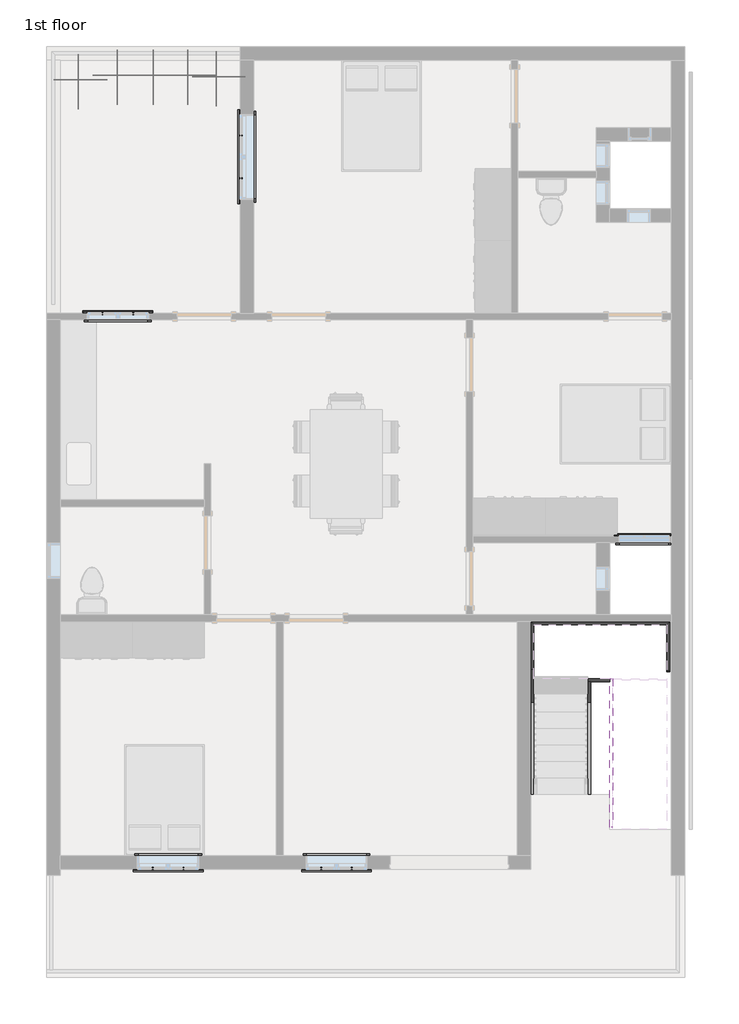
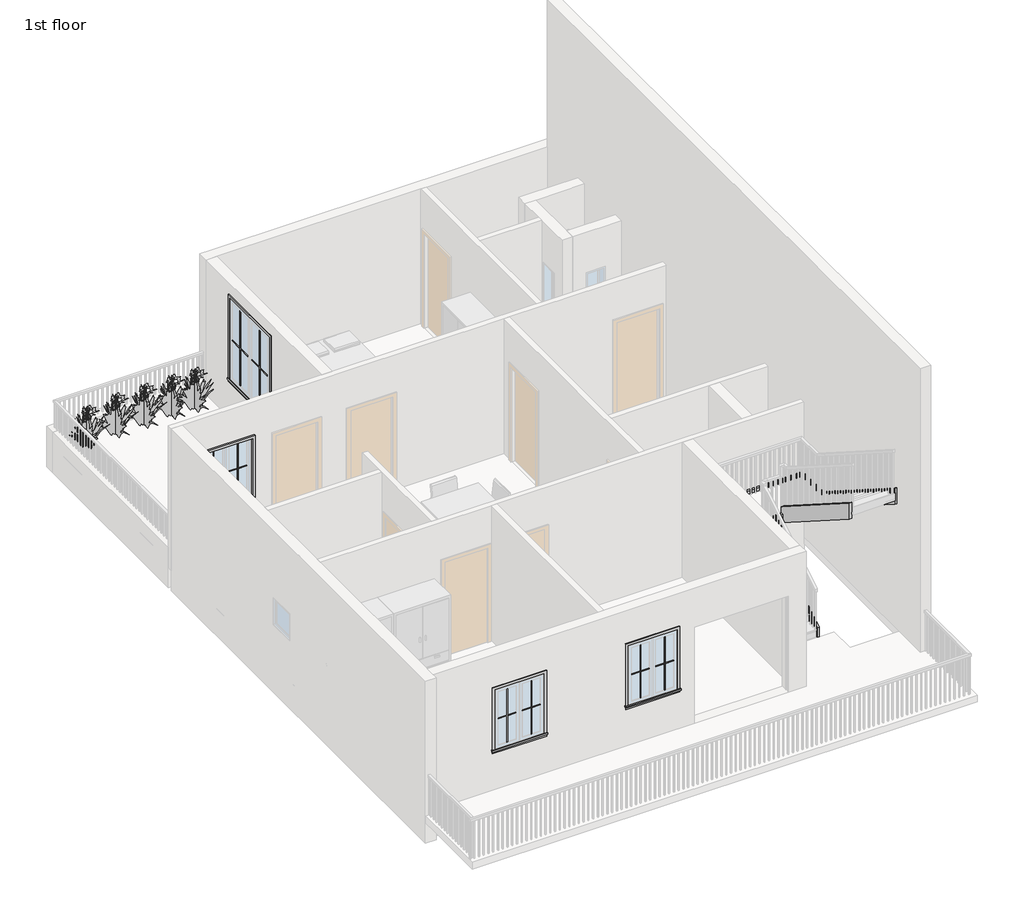
# One storey, part 5 of 5: 20 proxies, 8 members, 5 geographic elements.
"""IFC4 building model written with IfcOpenShell, lengths in millimetres."""

from ifc_helpers import new_model, si_unit, frame, origin, place, context, project, spatial, polyline, outline, extrude, faceted_brep, transform, mapped, element, save
from components import muntin_pattern_2x2_muntin_pattern_2x2_bff912c5, muntin_pattern_2x2_muntin_pattern_2x2_c2194282, muntin_pattern_2x2_muntin_pattern_2x2_88bf7f41, muntin_pattern_2x2_muntin_pattern_2x2_3dfd0a47, muntin_pattern_2x2_muntin_pattern_2x2_b3fe6957, muntin_pattern_2x2_muntin_pattern_2x2_3e0ecaf2, trim_window_exterior_flat_with_sill_e04b3088, trim_window_exterior_flat_with_sill_4930676f, trim_window_exterior_flat_with_sill_41619996, trim_window_interior_flat_picture_frame_2a7685fe, trim_window_interior_flat_picture_frame_dd064338, trim_window_interior_flat_picture_frame_51c85655, rpc_plant_tropical_55f6ff97

model = new_model("IFC4")

# Units and contexts
model_context = context("Model", 3, world=origin())
ifc_project = project(units=[si_unit("LENGTHUNIT", "METRE", prefix="MILLI")], contexts=[model_context])

# Site, building, storey
site = spatial("IfcSite", under=ifc_project)
building = spatial("IfcBuilding", under=site)
storey = spatial("IfcBuildingStorey", under=building, Name="1st floor", Elevation=3810.0)

# Proxies
placement = place(None, origin())
muntin_pattern_2x2_muntin_pattern_2x2_shape = muntin_pattern_2x2_muntin_pattern_2x2_bff912c5(model_context)
element("IfcBuildingElementProxy", 1, Name="Muntin Pattern_2x2 : Muntin Pattern_2x2", ObjectType="Muntin Pattern_2x2 : Muntin Pattern_2x2", at=placement, inside=storey, context=model_context, shape_type="MappedRepresentation", body=[
    mapped(muntin_pattern_2x2_muntin_pattern_2x2_shape, transform((-4824.2248597, 10579.5632925, 4794.25), x_axis=(0.0, 1.0, 0.0), y_axis=(-1.0, 0.0, 0.0), z_axis=(0.0, 0.0, 1.0))),
])
muntin_pattern_2x2_muntin_pattern_2x2_2_shape = muntin_pattern_2x2_muntin_pattern_2x2_c2194282(model_context)
element("IfcBuildingElementProxy", 2, Name="Muntin Pattern_2x2 : Muntin Pattern_2x2", ObjectType="Muntin Pattern_2x2 : Muntin Pattern_2x2", at=placement, inside=storey, context=model_context, shape_type="MappedRepresentation", body=[
    mapped(muntin_pattern_2x2_muntin_pattern_2x2_2_shape, transform((-4824.2248597, 11300.2882925, 4794.25), x_axis=(0.0, -1.0, 0.0), y_axis=(1.0, 0.0, 0.0), z_axis=(0.0, 0.0, 1.0))),
])
muntin_pattern_2x2_muntin_pattern_2x2_3_shape = muntin_pattern_2x2_muntin_pattern_2x2_88bf7f41(model_context)
element("IfcBuildingElementProxy", 3, Name="Muntin Pattern_2x2 : Muntin Pattern_2x2", ObjectType="Muntin Pattern_2x2 : Muntin Pattern_2x2", at=placement, inside=storey, context=model_context, shape_type="MappedRepresentation", body=[
    mapped(muntin_pattern_2x2_muntin_pattern_2x2_3_shape, transform((-7162.6123597, 8288.8007925, 4794.25), x_axis=(1.0, 0.0, 0.0), y_axis=(0.0, 1.0, 0.0), z_axis=(0.0, 0.0, 1.0))),
])
element("IfcBuildingElementProxy", 4, Name="Muntin Pattern_2x2 : Muntin Pattern_2x2", ObjectType="Muntin Pattern_2x2 : Muntin Pattern_2x2", at=placement, inside=storey, context=model_context, shape_type="MappedRepresentation", body=[
    mapped(muntin_pattern_2x2_muntin_pattern_2x2_3_shape, transform((-5794.1873597, -1102.8492075, 4794.25), x_axis=(-1.0, 0.0, 0.0), y_axis=(0.0, -1.0, 0.0), z_axis=(0.0, 0.0, 1.0))),
])
element("IfcBuildingElementProxy", 5, Name="Muntin Pattern_2x2 : Muntin Pattern_2x2", ObjectType="Muntin Pattern_2x2 : Muntin Pattern_2x2", at=placement, inside=storey, context=model_context, shape_type="MappedRepresentation", body=[
    mapped(muntin_pattern_2x2_muntin_pattern_2x2_3_shape, transform((-2946.0873597, -1102.8492075, 4794.25), x_axis=(-1.0, 0.0, 0.0), y_axis=(0.0, -1.0, 0.0), z_axis=(0.0, 0.0, 1.0))),
])
muntin_pattern_2x2_muntin_pattern_2x2_4_shape = muntin_pattern_2x2_muntin_pattern_2x2_3dfd0a47(model_context)
element("IfcBuildingElementProxy", 6, Name="Muntin Pattern_2x2 : Muntin Pattern_2x2", ObjectType="Muntin Pattern_2x2 : Muntin Pattern_2x2", at=placement, inside=storey, context=model_context, shape_type="MappedRepresentation", body=[
    mapped(muntin_pattern_2x2_muntin_pattern_2x2_4_shape, transform((-6645.0873597, 8288.8007925, 4794.25), x_axis=(-1.0, 0.0, 0.0), y_axis=(0.0, -1.0, 0.0), z_axis=(0.0, 0.0, 1.0))),
])
element("IfcBuildingElementProxy", 7, Name="Muntin Pattern_2x2 : Muntin Pattern_2x2", ObjectType="Muntin Pattern_2x2 : Muntin Pattern_2x2", at=placement, inside=storey, context=model_context, shape_type="MappedRepresentation", body=[
    mapped(muntin_pattern_2x2_muntin_pattern_2x2_4_shape, transform((-6311.7123597, -1102.8492075, 4794.25), x_axis=(1.0, 0.0, 0.0), y_axis=(0.0, 1.0, 0.0), z_axis=(0.0, 0.0, 1.0))),
])
element("IfcBuildingElementProxy", 8, Name="Muntin Pattern_2x2 : Muntin Pattern_2x2", ObjectType="Muntin Pattern_2x2 : Muntin Pattern_2x2", at=placement, inside=storey, context=model_context, shape_type="MappedRepresentation", body=[
    mapped(muntin_pattern_2x2_muntin_pattern_2x2_4_shape, transform((-3463.6123597, -1102.8492075, 4794.25), x_axis=(1.0, 0.0, 0.0), y_axis=(0.0, 1.0, 0.0), z_axis=(0.0, 0.0, 1.0))),
])
muntin_pattern_2x2_muntin_pattern_2x2_5_shape = muntin_pattern_2x2_muntin_pattern_2x2_b3fe6957(model_context)
element("IfcBuildingElementProxy", 9, Name="Muntin Pattern_2x2 : Muntin Pattern_2x2", ObjectType="Muntin Pattern_2x2 : Muntin Pattern_2x2", at=placement, inside=storey, context=model_context, shape_type="MappedRepresentation", body=[
    mapped(muntin_pattern_2x2_muntin_pattern_2x2_5_shape, transform((1784.5376403, 4516.9007925, 4184.65), x_axis=(1.0, 0.0, 0.0), y_axis=(0.0, 1.0, 0.0), z_axis=(0.0, 0.0, 1.0))),
])
muntin_pattern_2x2_muntin_pattern_2x2_6_shape = muntin_pattern_2x2_muntin_pattern_2x2_3e0ecaf2(model_context)
element("IfcBuildingElementProxy", 10, Name="Muntin Pattern_2x2 : Muntin Pattern_2x2", ObjectType="Muntin Pattern_2x2 : Muntin Pattern_2x2", at=placement, inside=storey, context=model_context, shape_type="MappedRepresentation", body=[
    mapped(muntin_pattern_2x2_muntin_pattern_2x2_6_shape, transform((2213.1626403, 4516.9007925, 4184.65), x_axis=(-1.0, 0.0, 0.0), y_axis=(0.0, -1.0, 0.0), z_axis=(0.0, 0.0, 1.0))),
])
trim_window_exterior_flat_with_sill_shape = trim_window_exterior_flat_with_sill_e04b3088(model_context)
element("IfcBuildingElementProxy", 11, Name="Trim-Window-Exterior-Flat : with Sill", ObjectType="Trim-Window-Exterior-Flat : with Sill", at=placement, inside=storey, context=model_context, shape_type="MappedRepresentation", body=[
    mapped(trim_window_exterior_flat_with_sill_shape, transform((-4833.7498597, 10939.9257925, 6553.2), x_axis=(0.0, -1.0, 0.0), y_axis=(0.0, 0.0, 1.0), z_axis=(-1.0, 0.0, 0.0))),
])
trim_window_exterior_flat_with_sill_2_shape = trim_window_exterior_flat_with_sill_4930676f(model_context)
element("IfcBuildingElementProxy", 12, Name="Trim-Window-Exterior-Flat : with Sill", ObjectType="Trim-Window-Exterior-Flat : with Sill", at=placement, inside=storey, context=model_context, shape_type="MappedRepresentation", body=[
    mapped(trim_window_exterior_flat_with_sill_2_shape, transform((-6903.8498597, 8298.3257925, 6070.6), x_axis=(-1.0, 0.0, 0.0), y_axis=(0.0, 0.0, 1.0), z_axis=(0.0, 1.0, 0.0))),
])
element("IfcBuildingElementProxy", 13, Name="Trim-Window-Exterior-Flat : with Sill", ObjectType="Trim-Window-Exterior-Flat : with Sill", at=placement, inside=storey, context=model_context, shape_type="MappedRepresentation", body=[
    mapped(trim_window_exterior_flat_with_sill_2_shape, transform((-6052.9498597, -1112.3742075, 6070.6), x_axis=(1.0, 0.0, 0.0), y_axis=(0.0, 0.0, 1.0), z_axis=(0.0, -1.0, 0.0))),
])
element("IfcBuildingElementProxy", 14, Name="Trim-Window-Exterior-Flat : with Sill", ObjectType="Trim-Window-Exterior-Flat : with Sill", at=placement, inside=storey, context=model_context, shape_type="MappedRepresentation", body=[
    mapped(trim_window_exterior_flat_with_sill_2_shape, transform((-3204.8498597, -1112.3742075, 6070.6), x_axis=(1.0, 0.0, 0.0), y_axis=(0.0, 0.0, 1.0), z_axis=(0.0, -1.0, 0.0))),
])
trim_window_exterior_flat_with_sill_3_shape = trim_window_exterior_flat_with_sill_41619996(model_context)
element("IfcBuildingElementProxy", 15, Name="Trim-Window-Exterior-Flat : with Sill", ObjectType="Trim-Window-Exterior-Flat : with Sill", at=placement, inside=storey, context=model_context, shape_type="MappedRepresentation", body=[
    mapped(trim_window_exterior_flat_with_sill_3_shape, transform((1998.8501403, 4526.4257925, 5029.2), x_axis=(-1.0, 0.0, 0.0), y_axis=(0.0, 0.0, 1.0), z_axis=(0.0, 1.0, 0.0))),
])
trim_window_interior_flat_picture_frame_shape = trim_window_interior_flat_picture_frame_2a7685fe(model_context)
element("IfcBuildingElementProxy", 16, Name="Trim-Window-Interior-Flat : Picture Frame", ObjectType="Trim-Window-Interior-Flat : Picture Frame", at=placement, inside=storey, context=model_context, shape_type="MappedRepresentation", body=[
    mapped(trim_window_interior_flat_picture_frame_shape, transform((-4605.1498597, 10939.9257925, 6553.2), x_axis=(0.0, 1.0, 0.0), y_axis=(0.0, 0.0, 1.0), z_axis=(1.0, 0.0, 0.0))),
])
trim_window_interior_flat_picture_frame_2_shape = trim_window_interior_flat_picture_frame_dd064338(model_context)
element("IfcBuildingElementProxy", 17, Name="Trim-Window-Interior-Flat : Picture Frame", ObjectType="Trim-Window-Interior-Flat : Picture Frame", at=placement, inside=storey, context=model_context, shape_type="MappedRepresentation", body=[
    mapped(trim_window_interior_flat_picture_frame_2_shape, transform((-6903.8498597, 8184.0257925, 6070.6), x_axis=(1.0, 0.0, 0.0), y_axis=(0.0, 0.0, 1.0), z_axis=(0.0, -1.0, 0.0))),
])
element("IfcBuildingElementProxy", 18, Name="Trim-Window-Interior-Flat : Picture Frame", ObjectType="Trim-Window-Interior-Flat : Picture Frame", at=placement, inside=storey, context=model_context, shape_type="MappedRepresentation", body=[
    mapped(trim_window_interior_flat_picture_frame_2_shape, transform((-6052.9498597, -883.7742075, 6070.6), x_axis=(-1.0, 0.0, 0.0), y_axis=(0.0, 0.0, 1.0), z_axis=(0.0, 1.0, 0.0))),
])
element("IfcBuildingElementProxy", 19, Name="Trim-Window-Interior-Flat : Picture Frame", ObjectType="Trim-Window-Interior-Flat : Picture Frame", at=placement, inside=storey, context=model_context, shape_type="MappedRepresentation", body=[
    mapped(trim_window_interior_flat_picture_frame_2_shape, transform((-3204.8498597, -883.7742075, 6070.6), x_axis=(-1.0, 0.0, 0.0), y_axis=(0.0, 0.0, 1.0), z_axis=(0.0, 1.0, 0.0))),
])
trim_window_interior_flat_picture_frame_3_shape = trim_window_interior_flat_picture_frame_51c85655(model_context)
element("IfcBuildingElementProxy", 20, Name="Trim-Window-Interior-Flat : Picture Frame", ObjectType="Trim-Window-Interior-Flat : Picture Frame", at=placement, inside=storey, context=model_context, shape_type="MappedRepresentation", body=[
    mapped(trim_window_interior_flat_picture_frame_3_shape, transform((1998.8501403, 4412.1257925, 5029.2), x_axis=(1.0, 0.0, 0.0), y_axis=(0.0, 0.0, 1.0), z_axis=(0.0, -1.0, 0.0))),
])

# Geographic elements
rpc_plant_tropical_shape = rpc_plant_tropical_55f6ff97(model_context)
element("IfcGeographicElement", 21, ObjectType="RPC Plant - Tropical", at=placement, inside=storey, context=model_context, shape_type="MappedRepresentation", body=[
    mapped(rpc_plant_tropical_shape, transform((-7576.9498597, 12248.0257925, 3810.0), x_axis=(1.0, 0.0, 0.0), y_axis=(0.0, 1.0, 0.0), z_axis=(0.0, 0.0, 1.0))),
])
element("IfcGeographicElement", 22, ObjectType="RPC Plant - Tropical", at=placement, inside=storey, context=model_context, shape_type="MappedRepresentation", body=[
    mapped(rpc_plant_tropical_shape, transform((-5240.1498597, 12298.8257925, 3810.0), x_axis=(1.0, 0.0, 0.0), y_axis=(0.0, 1.0, 0.0), z_axis=(0.0, 0.0, 1.0))),
])
element("IfcGeographicElement", 23, ObjectType="RPC Plant - Tropical", at=placement, inside=storey, context=model_context, shape_type="MappedRepresentation", body=[
    mapped(rpc_plant_tropical_shape, transform((-6916.5498597, 12324.2257925, 3810.0), x_axis=(1.0, 0.0, 0.0), y_axis=(0.0, 1.0, 0.0), z_axis=(0.0, 0.0, 1.0))),
])
element("IfcGeographicElement", 24, ObjectType="RPC Plant - Tropical", at=placement, inside=storey, context=model_context, shape_type="MappedRepresentation", body=[
    mapped(rpc_plant_tropical_shape, transform((-6306.9498597, 12324.2257925, 3810.0), x_axis=(1.0, 0.0, 0.0), y_axis=(0.0, 1.0, 0.0), z_axis=(0.0, 0.0, 1.0))),
])
element("IfcGeographicElement", 25, ObjectType="RPC Plant - Tropical", at=placement, inside=storey, context=model_context, shape_type="MappedRepresentation", body=[
    mapped(rpc_plant_tropical_shape, transform((-5722.7498597, 12324.2257925, 3810.0), x_axis=(1.0, 0.0, 0.0), y_axis=(0.0, 1.0, 0.0), z_axis=(0.0, 0.0, 1.0))),
])

# Members
element("IfcMember", 26, ObjectType="Stringer - 2\" Width", at=placement, inside=storey, context=model_context, shape_type="SweptSolid", body=[
    extrude(outline(polyline([(157.6257925, 3810.0), (157.6257925, 4025.0106437), (2174.694781, 5308.6), (2263.4527505, 5003.8), (387.4813219, 3810.0), (157.6257925, 3810.0)])), frame((81.1501403, 0.0, 0.0), z_axis=(1.0, 0.0, 0.0), x_axis=(0.0, 1.0, 0.0)), (0.0, 0.0, 1.0), 50.8),
])
element("IfcMember", 27, ObjectType="Stringer - 2\" Width", at=placement, inside=storey, context=model_context, shape_type="SweptSolid", body=[
    extrude(outline(polyline([(157.6257925, 3810.0), (157.6257925, 4025.0106437), (2062.6257925, 5237.283371), (2062.6257925, 4876.0010268), (387.4813219, 3810.0), (157.6257925, 3810.0)])), frame((1046.3501403, 0.0, 0.0), z_axis=(1.0, 0.0, 0.0), x_axis=(0.0, 1.0, 0.0)), (0.0, 0.0, 1.0), 50.8),
])
element("IfcMember", 28, ObjectType="Stringer - 2\" Width", at=placement, inside=storey, context=model_context, shape_type="SweptSolid", body=[
    extrude(outline(polyline([(2331.5568041, 5308.6), (2242.7988346, 5003.8), (-401.1742075, 6686.3282995), (-401.1742075, 7047.6106437), (2331.5568041, 5308.6)])), frame((2379.8501403, 0.0, 0.0), z_axis=(1.0, 0.0, 0.0), x_axis=(0.0, 1.0, 0.0)), (0.0, 0.0, 1.0), 50.8),
])
element("IfcMember", 29, ObjectType="Stringer - 2\" Width", at=placement, inside=storey, context=model_context, shape_type="SweptSolid", body=[
    extrude(outline(polyline([(2113.4257925, 5447.4106437), (2113.4257925, 5086.1282995), (-401.1742075, 6686.3282995), (-401.1742075, 7047.6106437), (2113.4257925, 5447.4106437)])), frame((1414.6501403, 0.0, 0.0), z_axis=(1.0, 0.0, 0.0), x_axis=(0.0, 1.0, 0.0)), (0.0, 0.0, 1.0), 50.8),
])
element("IfcMember", 30, ObjectType="Stringer - 2\" Width", at=placement, inside=storey, context=model_context, shape_type="Brep", body=[
    faceted_brep([(2379.8501403, 2331.5568041, 5308.6), (2430.6501403, 2331.5568041, 5308.6), (2430.6501403, 3078.6257925, 5308.6), (2379.8501403, 3027.8257925, 5308.6), (2379.8501403, 2242.7988346, 5003.8), (2379.8501403, 3027.8257925, 5003.8), (2430.6501403, 2242.7988346, 5003.8), (2430.6501403, 3078.6257925, 5003.8)], [[[0, 1, 2, 3]], [[4, 0, 3, 5]], [[6, 4, 5, 7]], [[1, 6, 7, 2]], [[1, 0, 4, 6]], [[2, 7, 5, 3]]]),
])
element("IfcMember", 31, ObjectType="Stringer - 2\" Width", at=placement, inside=storey, context=model_context, shape_type="SweptSolid", body=[
    extrude(outline(polyline([(2430.6501403, 3078.6257925), (2379.8501403, 3027.8257925), (131.9501403, 3027.8257925), (81.1501403, 3078.6257925), (2430.6501403, 3078.6257925)])), frame((0.0, 0.0, 5003.8), z_axis=(0.0, 0.0, 1.0), x_axis=(1.0, 0.0, 0.0)), (0.0, 0.0, 1.0), 304.8),
])
element("IfcMember", 32, ObjectType="Stringer - 2\" Width", at=placement, inside=storey, context=model_context, shape_type="Brep", body=[
    faceted_brep([(131.9501403, 3027.8257925, 5308.6), (81.1501403, 3078.6257925, 5308.6), (81.1501403, 2174.694781, 5308.6), (131.9501403, 2174.694781, 5308.6), (131.9501403, 3027.8257925, 5003.8), (131.9501403, 2263.4527505, 5003.8), (81.1501403, 3078.6257925, 5003.8), (81.1501403, 2263.4527505, 5003.8)], [[[0, 1, 2, 3]], [[4, 0, 3, 5]], [[6, 4, 5, 7]], [[1, 6, 7, 2]], [[1, 0, 4, 6]], [[2, 7, 5, 3]]]),
])
element("IfcMember", 33, ObjectType="Stringer - 2\" Width", at=placement, inside=storey, context=model_context, shape_type="SweptSolid", body=[
    extrude(outline(polyline([(1046.3501403, 2062.6257925), (1046.3501403, 2113.4257925), (1414.6501403, 2113.4257925), (1414.6501403, 2062.6257925), (1046.3501403, 2062.6257925)])), frame((0.0, 0.0, 5003.8), z_axis=(0.0, 0.0, 1.0), x_axis=(1.0, 0.0, 0.0)), (0.0, 0.0, 1.0), 304.8),
])

save(model, "model.ifc")

# Revit data of these elements
# Type "Muntin Pattern_2x2 : Muntin Pattern_2x2"
#   Width [instance default] = 4' - 0"
#   Thickness = 0' - 0 1/2"
#   Height [instance default] = 4' - 0"
#   Distance = 0' - 0 3/4"
#   Interior Material [instance default] = none
#   Exterior Material [instance default] = none
#   Default Elevation = 0
# Type "Trim-Window-Exterior-Flat : with Sill"
#   Trim Width = 0' - 2 1/4"
#   Trim Thickness_Picture Frame = 0' - 1 1/4"
#   Trim Thickness_with Sill = 0' - 0 3/4"
#   Sill Thickness = 0' - 1 1/4"
#   Opening Width [instance default] = 2' - 0"
#   Opening Height [instance default] = 3' - 0"
#   Default Elevation = 4' - 0"
#   Sill = yes
#   Picture Frame = no
#   Trim Material [instance default] = none
# Type "Trim-Window-Interior-Flat : Picture Frame"
#   Trim Thickness_Picture Frame = 0' - 1 1/4"
#   Trim Width = 0' - 2 1/4"
#   Trim Thickness_with Sill = 0' - 0 3/4"
#   Sill Thickness = 0' - 1 1/4"
#   Opening Width [instance default] = 2' - 0"
#   Opening Height [instance default] = 3' - 0"
#   Default Elevation = 4' - 0"
#   Sill = no
#   Picture Frame = yes
#   Trim Material [instance default] = none
# Type "RPC Plant - Tropical"
#   built-in parameter 1005198 = "{2, 15},{39, RPC-16-FWM5-GM7X-C67P-4000-ST1L-LVER-AU},{1, 0},{1, 0},{2, 35},{1, 8},{5, Color},{1, 0},{1, 0},{3, 0.8},{3, 0.8},{3, 0.8},{1, 8},{7, BBoxMin},{1, 0},{1, 0},{1, 0},{1, 0},{1, 0},{1, 8},{7, BBoxMax},{1, 0},{1, 0},{1, 0},{1, 0},{1, 0},{2, 11},{9, RPCTypeId},{1, 0},{1, 0},{39, RPC-16-FWM5-GM7X-C67P-4000-ST1L-LVER-AU},{1, 6},{14, RPCPlantHeight},{1, 0},{1, 0},{1, 3},{2, 11},{7, keyword},{1, 0},{1, 0},{99, :Geometry:RPC:Crane Lily:strelitzia:reinae:crane lily:plants:shrub:flower:tropical:bird-of-paradise},{2, 11},{8, category},{1, 0},{1, 0},{17, :Shrubs [General]},{2, 11},{12, LocalizedUID},{1, 0},{1, 0},{10, Crane Lily},{2, 14},{6, Height},{1, 0},{1, 0},{1, 3},{1, 2},{16, Cast Reflections},{1, 0},{1, 0},{1, 0},{1, 2},{12, Cast Shadows},{1, 0},{1, 0},{1, 1},{1, 2},{9, Lock View},{1, 0},{1, 0},{1, 0},{1, 4},{5, ViewC},{1, 0},{1, 0},{1, 0},{2, 11},{20, AdvancedUIDefinition},{1, 0},{1, 0},{0, },{2, 11},{10, AssetLibID},{1, 0},{1, 0},{36, 4D3F6E72-3F99-4203-98E9-AF80B3C7A7A4},{2, 11},{10, BaseSchema},{1, 0},{1, 0},{9, RPCSchema},{2, 11},{12, ExchangeGUID},{1, 0},{1, 0},{0, },{1, 2},{6, Hidden},{1, 0},{1, 0},{1, 0},{1, 4},{11, RPCCategory},{1, 0},{1, 0},{1, 0},{2, 11},{8, RPCImage},{1, 0},{1, 0},{0, },{1, 4},{13, SchemaVersion},{1, 0},{1, 0},{1, 4},{2, 11},{12, UIDefinition},{1, 0},{1, 0},{0, },{2, 11},{6, UIName},{1, 0},{1, 0},{39, RPC-16-FWM5-GM7X-C67P-4000-ST1L-LVER-AU},{2, 11},{11, VersionGUID},{1, 0},{1, 0},{9, RPCSchema},{2, 11},{9, assettype},{1, 0},{1, 0},{11, RPCGeometry},{2, 11},{11, description},{1, 0},{1, 0},{0, },{2, 11},{9, localname},{1, 0},{1, 0},{3, RPC},{2, 11},{9, localtype},{1, 0},{1, 0},{3, RPC},{1, 4},{8, revision},{1, 0},{1, 0},{1, 1},{2, 11},{9, thumbnail},{1, 0},{1, 0},{0, },{1, 4},{7, version},{1, 0},{1, 0},{1, 1},{1, 2},{20, RPC_Cast Reflections},{1, 0},{1, 0},{1, 1},{1, 2},{16, RPC_Cast Shadows},{1, 0},{1, 0},{1, 1},{1, 2},{13, RPC_Lock View},{1, 0},{1, 0},{1, 0},{1, 4},{9, RPC_ViewC},{1, 0},{1, 0},{1, 0},{21, assetlibrary_base.fbx},{1, 5},"
#   built-in parameter 1005195 = "RPC-16-FWM5-GM7X-C67P-4000-ST1L-LVER-AU"
#   Assembly Code = "G2050500"
#   Height = 3' - 0"
#   Default Elevation = 0
# Elements 1, 2 (IfcBuildingElementProxy, "Muntin Pattern_2x2 : Muntin Pattern_2x2")
#   Width = 1' - 11 1/8"
#   Height = 5' - 6 1/2"
#   Interior Material = Wood - Stained
#   Exterior Material = Clad - White
#   Phase Created = New Construction
#   Materials on its faces: "Clad - White", "Wood - Stained"
# Elements 3, 4, 5, 6, 7, 8 (IfcBuildingElementProxy, "Muntin Pattern_2x2 : Muntin Pattern_2x2")
#   Width = 1' - 3 1/8"
#   Height = 3' - 11 1/2"
#   Interior Material = Wood - Stained
#   Exterior Material = Clad - White
#   Phase Created = New Construction
#   Materials on its faces: "Clad - White", "Wood - Stained"
# Elements 9, 10 (IfcBuildingElementProxy, "Muntin Pattern_2x2 : Muntin Pattern_2x2")
#   Width = 0' - 11 5/8"
#   Height = 2' - 6 1/2"
#   Interior Material = Wood - Stained
#   Exterior Material = Clad - White
#   Phase Created = New Construction
#   Materials on its faces: "Clad - White", "Wood - Stained"
# Element 11 (IfcBuildingElementProxy, "Trim-Window-Exterior-Flat : with Sill")
#   Opening Width = 4' - 9"
#   Opening Height = 6' - 0"
#   Trim Material = Clad - White
#   Phase Created = New Construction
#   Materials on its faces: "Clad - White"
# Elements 12, 13, 14 (IfcBuildingElementProxy, "Trim-Window-Exterior-Flat : with Sill")
#   Opening Width = 3' - 5"
#   Opening Height = 4' - 5"
#   Trim Material = Clad - White
#   Phase Created = New Construction
#   Materials on its faces: "Clad - White"
# Element 15 (IfcBuildingElementProxy, "Trim-Window-Exterior-Flat : with Sill")
#   Opening Width = 2' - 10"
#   Opening Height = 3' - 0"
#   Trim Material = Clad - White
#   Phase Created = New Construction
#   Materials on its faces: "Clad - White"
# Element 16 (IfcBuildingElementProxy, "Trim-Window-Interior-Flat : Picture Frame")
#   Opening Width = 4' - 9"
#   Opening Height = 6' - 0"
#   Trim Material = Wood - Stained
#   Phase Created = New Construction
#   Materials on its faces: "Wood - Stained"
# Elements 17, 18, 19 (IfcBuildingElementProxy, "Trim-Window-Interior-Flat : Picture Frame")
#   Opening Width = 3' - 5"
#   Opening Height = 4' - 5"
#   Trim Material = Wood - Stained
#   Phase Created = New Construction
#   Materials on its faces: "Wood - Stained"
# Element 20 (IfcBuildingElementProxy, "Trim-Window-Interior-Flat : Picture Frame")
#   Opening Width = 2' - 10"
#   Opening Height = 3' - 0"
#   Trim Material = Wood - Stained
#   Phase Created = New Construction
#   Materials on its faces: "Wood - Stained"
# Elements 21, 22, 23, 24, 25 (IfcGeographicElement, "RPC Plant - Tropical")
#   Phase Created = New Construction
# Elements 26, 27, 28, 29, 30, 31, 32, 33 (IfcMember, "Stringer - 2\" Width")
#   Phase Created = New Construction
# Materials
#   "Clad - White": class "Wood", colour RGB 242 242 238, transparency 0, Cost = 0
#   "Wood - Stained": class "Wood", colour RGB 224 178 126, transparency 0, Cost = 0
